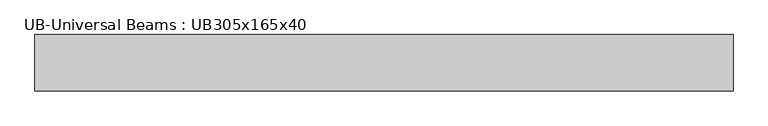
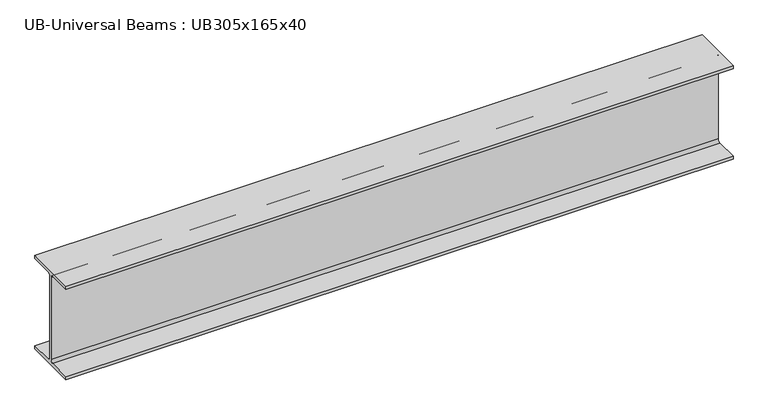
"""IFC4 building model written with IfcOpenShell, lengths in millimetres: beam geometry, UB-Universal Beams : UB305x165x40."""

from ifc_helpers import new_model, si_unit, point, frame, frame_2d, origin, place, context, project, spatial, polyline, circle_curve, trimmed, segment, composite_curve, outline, extrude, source, transform, mapped, element, save


def ub_universal_beams_ub305x165x40_fd314e36(model_context):
    return source(origin(), model_context, "Body", "SweptSolid", [
        extrude(outline(composite_curve([segment(polyline([(82.5, -141.5), (82.5, -151.7), (-82.5, -151.7), (-82.5, -141.5), (-11.9, -141.5)]), True, "CONTINUOUS"), segment(trimmed(circle_curve(frame_2d((-11.9, -132.6)), 8.9), [point((-11.9, -141.5))], [point((-3.0, -132.6))], True, "CARTESIAN"), True, "CONTINUOUS"), segment(polyline([(-3.0, -132.6), (-3.0, 132.6)]), True, "CONTINUOUS"), segment(trimmed(circle_curve(frame_2d((-11.9, 132.6)), 8.9), [point((-3.0, 132.6))], [point((-11.9, 141.5))], True, "CARTESIAN"), True, "CONTINUOUS"), segment(polyline([(-11.9, 141.5), (-82.5, 141.5), (-82.5, 151.7), (82.5, 151.7), (82.5, 141.5), (11.9, 141.5)]), True, "CONTINUOUS"), segment(trimmed(circle_curve(frame_2d((11.9, 132.6)), 8.9), [point((11.9, 141.5))], [point((3.0, 132.6))], True, "CARTESIAN"), True, "CONTINUOUS"), segment(polyline([(3.0, 132.6), (3.0, -132.6)]), True, "CONTINUOUS"), segment(trimmed(circle_curve(frame_2d((11.9, -132.6)), 8.9), [point((3.0, -132.6))], [point((11.9, -141.5))], True, "CARTESIAN"), True, "CONTINUOUS"), segment(polyline([(11.9, -141.5), (82.5, -141.5)]), True, "CONTINUOUS")], self_intersect=False)), frame((-1035.6, 0.0, 0.0), z_axis=(1.0, 0.0, 0.0), x_axis=(0.0, 1.0, 0.0)), (0.0, 0.0, 1.0), 2045.4),
    ])


if __name__ == "__main__":
    model = new_model("IFC4")
    model_context = context("Model", 3, world=origin())
    ifc_project = project(units=[si_unit("LENGTHUNIT", "METRE", prefix="MILLI")], contexts=[model_context])
    site = spatial("IfcSite", under=ifc_project)
    building = spatial("IfcBuilding", under=site)
    placement = place(None, origin())
    ub_universal_beams_ub305x165x40_shape = ub_universal_beams_ub305x165x40_fd314e36(model_context)
    element("IfcBeam", 1, ObjectType="UB-Universal Beams : UB305x165x40", at=placement, inside=building, context=model_context, shape_type="MappedRepresentation", body=[
        mapped(ub_universal_beams_ub305x165x40_shape, transform((0.0, 0.0, 0.0), x_axis=(1.0, 0.0, 0.0), y_axis=(0.0, 1.0, 0.0), z_axis=(0.0, 0.0, 1.0))),
    ])
    save(model, "model.ifc")

# Revit data of these elements
# Type "UB-Universal Beams : UB305x165x40"
#   Section Name Key = "UB305X165X40"
#   Width = 16.5 cm
#   Web Thickness = 0.6 cm
#   Web Fillet = 0.89 cm
#   Warping Constant = 164000.0 cm⁶
#   Torsional Moment of Inertia = 14.70 cm⁴
#   Section Area = 51.3 cm²
#   Plastic Modulus weak axis = 142.0 cm³
#   Plastic Modulus strong axis = 623.0 cm³
#   Nominal Weight = 40.2999 kgf/m
#   Moment of Inertia weak axis = 764.00 cm⁴
#   Moment of Inertia strong axis = 8503.00 cm⁴
#   Height = 30.34 cm
#   Flange Thickness = 1.02 cm
#   Elastic Modulus weak axis = 92.6 cm³
#   Elastic Modulus strong axis = 560.0 cm³
#   Centroid Vertical = 15.17 cm
#   Centroid Horizontal = 8.25 cm
#   Bolt Spacing = 9.0 cm
#   Length [instance default] = 1500 mm
#   Structural Material [instance default] = Metal - Steel 43-275
#   Type Comments = ""
#   Assembly Code = ""
# Element 1 (IfcBeam, "UB-Universal Beams : UB305x165x40")
#   Materials on its faces: "Metal - Steel 43-275"
# Materials
#   "Metal - Steel 43-275": class "Metal", colour RGB 247 247 247, transparency 0, Cost = 0
